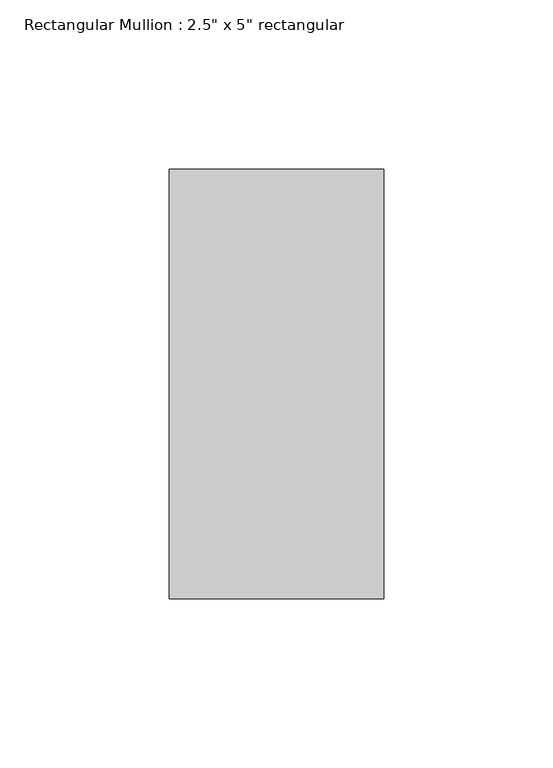
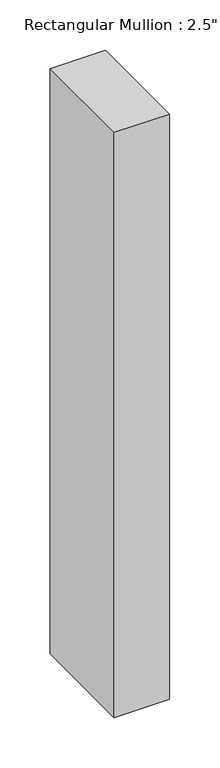
"""IFC4 building model written with IfcOpenShell, lengths in millimetres: member geometry."""

from ifc_helpers import new_model, si_unit, frame, origin, place, context, project, spatial, polyline, outline, extrude, source, transform, mapped, element, save


def member_df93ad89(model_context):
    return source(origin(), model_context, "Body", "SweptSolid", [
        extrude(outline(polyline([(0.0, 63.5), (0.0, -63.5), (-63.5, -63.5), (-63.5, 63.5), (0.0, 63.5)])), frame((0.0, 0.0, -708.4612955), z_axis=(0.0, 0.0, 1.0), x_axis=(1.0, 0.0, 0.0)), (0.0, 0.0, 1.0), 708.4612955),
    ])


if __name__ == "__main__":
    model = new_model("IFC4")
    model_context = context("Model", 3, world=origin())
    ifc_project = project(units=[si_unit("LENGTHUNIT", "METRE", prefix="MILLI")], contexts=[model_context])
    site = spatial("IfcSite", under=ifc_project)
    building = spatial("IfcBuilding", under=site)
    placement = place(None, origin())
    member_shape = member_df93ad89(model_context)
    element("IfcMember", 1, ObjectType="Rectangular Mullion : 2.5\" x 5\" rectangular", at=placement, inside=building, context=model_context, shape_type="MappedRepresentation", body=[
        mapped(member_shape, transform((0.0, 0.0, 0.0), x_axis=(1.0, 0.0, 0.0), y_axis=(0.0, 1.0, 0.0), z_axis=(0.0, 0.0, 1.0))),
    ])
    save(model, "model.ifc")

# Revit data of these elements
# Type "Rectangular Mullion : 2.5\" x 5\" rectangular"
#   built-in parameter 1007304 = 0.416667 (stored number, unit not read)
#   built-in parameter 1007301 = 0.104167 (stored number, unit not read)
#   built-in parameter 1007300 = 0.104167 (stored number, unit not read)
# Element 1 (IfcMember, "Rectangular Mullion : 2.5\" x 5\" rectangular")
#   Materials on its faces: "Aluminum"
# Materials
#   "Aluminum": class "Metal", colour RGB 247 247 247, transparency 0, Description = "Aluminum 6061", Cost = 0
